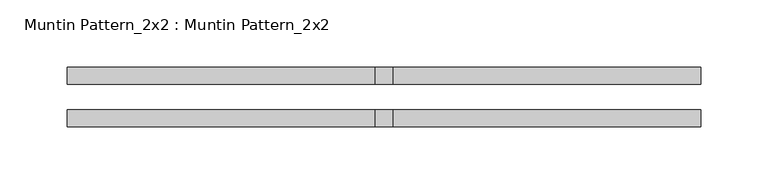
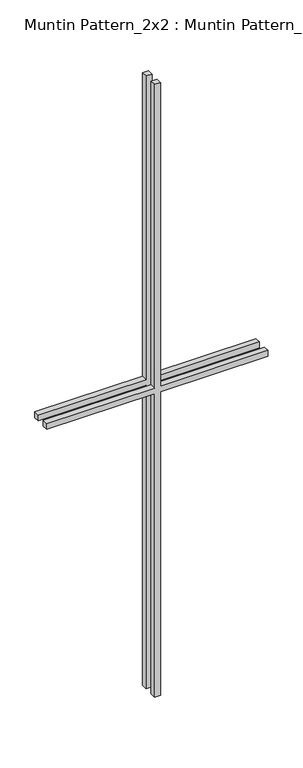
"""IFC4 building model written with IfcOpenShell, lengths in millimetres: proxy geometry, Muntin Pattern_2x2 : Muntin Pattern_2x2."""

from ifc_helpers import new_model, si_unit, frame, origin, place, context, project, spatial, polyline, outline, extrude, source, transform, mapped, element, save


def muntin_pattern_2x2_muntin_pattern_2x2_6dad3731(model_context):
    return source(origin(), model_context, "Body", "SweptSolid", [
        extrude(outline(polyline([(698.5, -6.35), (698.5, -236.5375), (685.8, -236.5375), (685.8, -6.35), (0.0, -6.35), (0.0, 6.35), (685.8, 6.35), (685.8, 236.5375), (698.5, 236.5375), (698.5, 6.35), (1384.3, 6.35), (1384.3, -6.35), (698.5, -6.35)])), frame((0.0, 9.525, 0.0), z_axis=(0.0, 1.0, 0.0), x_axis=(0.0, 0.0, 1.0)), (0.0, 0.0, 1.0), 12.7),
        extrude(outline(polyline([(698.5, -6.35), (698.5, -236.5375), (685.8, -236.5375), (685.8, -6.35), (0.0, -6.35), (0.0, 6.35), (685.8, 6.35), (685.8, 236.5375), (698.5, 236.5375), (698.5, 6.35), (1384.3, 6.35), (1384.3, -6.35), (698.5, -6.35)])), frame((0.0, -22.225, 0.0), z_axis=(0.0, 1.0, 0.0), x_axis=(0.0, 0.0, 1.0)), (0.0, 0.0, 1.0), 12.7),
    ])


if __name__ == "__main__":
    model = new_model("IFC4")
    model_context = context("Model", 3, world=origin())
    ifc_project = project(units=[si_unit("LENGTHUNIT", "METRE", prefix="MILLI")], contexts=[model_context])
    site = spatial("IfcSite", under=ifc_project)
    building = spatial("IfcBuilding", under=site)
    placement = place(None, origin())
    muntin_pattern_2x2_muntin_pattern_2x2_shape = muntin_pattern_2x2_muntin_pattern_2x2_6dad3731(model_context)
    element("IfcBuildingElementProxy", 1, Name="Muntin Pattern_2x2 : Muntin Pattern_2x2", ObjectType="Muntin Pattern_2x2 : Muntin Pattern_2x2", at=placement, inside=building, context=model_context, shape_type="MappedRepresentation", body=[
        mapped(muntin_pattern_2x2_muntin_pattern_2x2_shape, transform((0.0, 0.0, 0.0), x_axis=(1.0, 0.0, 0.0), y_axis=(0.0, 1.0, 0.0), z_axis=(0.0, 0.0, 1.0))),
    ])
    save(model, "model.ifc")

# Revit data of these elements
# Type "Muntin Pattern_2x2 : Muntin Pattern_2x2"
#   Width [instance default] = 4' - 0"
#   Thickness = 0' - 0 1/2"
#   Height [instance default] = 4' - 0"
#   Distance = 0' - 0 3/4"
#   Interior Material [instance default] = none
#   Exterior Material [instance default] = none
#   Default Elevation = 0
# Element 1 (IfcBuildingElementProxy, "Muntin Pattern_2x2 : Muntin Pattern_2x2")
#   Width = 1' - 6 5/8"
#   Height = 4' - 6 1/2"
#   Interior Material = Wood - Stained
#   Exterior Material = Clad - White
#   Materials on its faces: "Clad - White", "Wood - Stained"
# Materials
#   "Clad - White": class "Wood", colour RGB 245 245 243, transparency 0, Cost = 0
#   "Wood - Stained": class "Wood", colour RGB 173 132 96, transparency 0, Cost = 0
